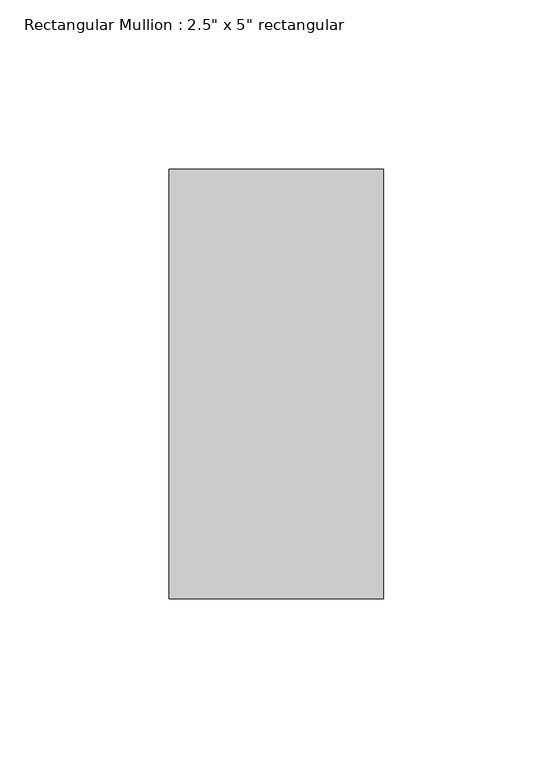
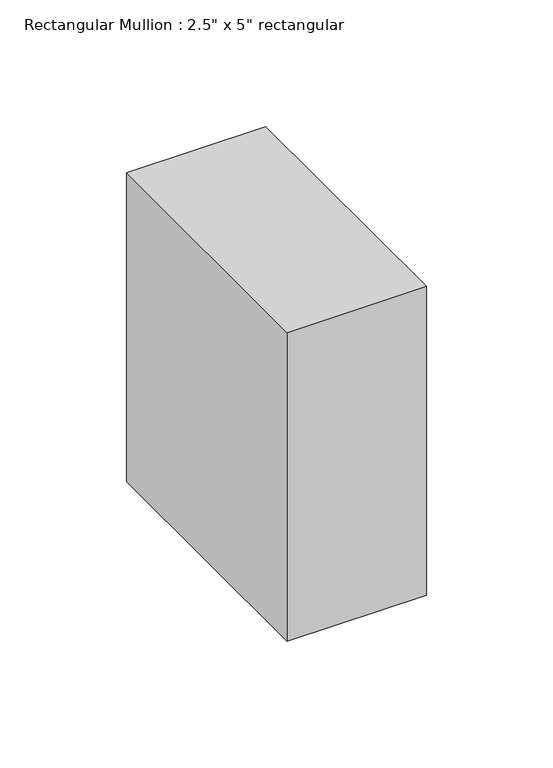
"""IFC4 building model written with IfcOpenShell, lengths in millimetres: member geometry."""

from ifc_helpers import new_model, si_unit, frame, origin, place, context, project, spatial, polyline, outline, extrude, source, transform, mapped, element, save


def member_c9ff5349(model_context):
    return source(origin(), model_context, "Body", "SweptSolid", [
        extrude(outline(polyline([(0.0, 63.5), (0.0, -63.5), (-63.5, -63.5), (-63.5, 63.5), (0.0, 63.5)])), frame((0.0, 0.0, -148.8191055), z_axis=(0.0, 0.0, 1.0), x_axis=(1.0, 0.0, 0.0)), (0.0, 0.0, 1.0), 148.8191055),
    ])


if __name__ == "__main__":
    model = new_model("IFC4")
    model_context = context("Model", 3, world=origin())
    ifc_project = project(units=[si_unit("LENGTHUNIT", "METRE", prefix="MILLI")], contexts=[model_context])
    site = spatial("IfcSite", under=ifc_project)
    building = spatial("IfcBuilding", under=site)
    placement = place(None, origin())
    member_shape = member_c9ff5349(model_context)
    element("IfcMember", 1, ObjectType="Rectangular Mullion : 2.5\" x 5\" rectangular", at=placement, inside=building, context=model_context, shape_type="MappedRepresentation", body=[
        mapped(member_shape, transform((0.0, 0.0, 0.0), x_axis=(1.0, 0.0, 0.0), y_axis=(0.0, 1.0, 0.0), z_axis=(0.0, 0.0, 1.0))),
    ])
    save(model, "model.ifc")

# Revit data of these elements
# Type "Rectangular Mullion : 2.5\" x 5\" rectangular"
#   built-in parameter 1007304 = 0.416667 (stored number, unit not read)
#   built-in parameter 1007301 = 0.104167 (stored number, unit not read)
#   built-in parameter 1007300 = 0.104167 (stored number, unit not read)
# Element 1 (IfcMember, "Rectangular Mullion : 2.5\" x 5\" rectangular")
#   Materials on its faces: "WINDOW FRAMING"
# Materials
#   "WINDOW FRAMING": class "Generic", colour RGB 120 120 120, transparency 0, Cost = 0
